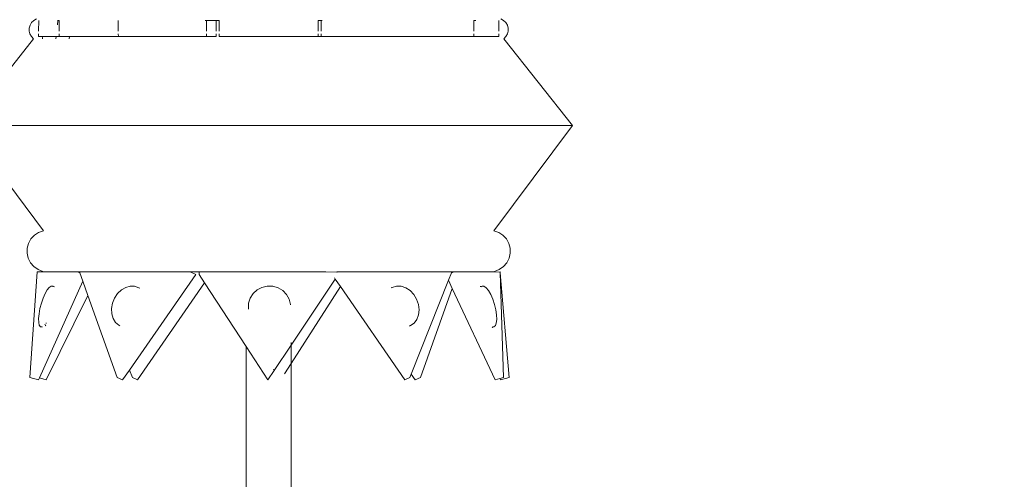
# Model space of a CAD drawing. Units: millimetres. Extents: x 7894 to 8038, y 6851 to 6951.
# Tile 39 of 49: x 7969.515 to 7972.111, y 6925.542 to 6926.755. Entities that reach past the tile are written whole.
import ezdxf

# ---------------------------------------------------------------- set-up
doc = ezdxf.new("R2010")
doc.units = ezdxf.units.MM
doc.layers.add('A-ANNO-DIMS', color=2, linetype='Continuous', lineweight=18)
doc.layers.add('A-FURN-ACCS', color=8, linetype='Continuous', lineweight=13)
doc.styles.get("Standard").update_dxf_attribs({"font": 'arial.ttf'})
doc.dimstyles.new('ISO-25', dxfattribs={"dimtxt": 1, "dimasz": 1, "dimexe": 1.25, "dimexo": 0.625, "dimtad": 1, "dimdec": 0, "dimlunit": 4, "dimtxsty": 'Standard', "dimcen": 2.5, "dimclrt": 1, "dimadec": 0, "dimazin": 0, "dimtfac": 1, "dimtdec": 0, "dimtmove": 0, "dimatfit": 3, "dimfxl": 1, "dimarcsym": 0})

# ---------------------------------------------------------------- blocks, each defined once
blk = doc.blocks.new('DISPLAY-LEAF-FINIAL-Z2_152')
for p, q in [((0.1759, 1.892, 2.1518), (0.1817, 1.8976, 2.1518)), ((0.1817, 1.8976, 2.1518), (0.1886, 1.9015, 2.1518)), ((0.1946, 1.8976, 2.1518), (0.1945, 1.8695, 2.1518)), ((0.2453, 1.8976, 2.1518), (0.2439, 1.8856, 2.1518)), ((0.2485, 1.8971, 2.1518), (0.2439, 1.8971, 2.1518)), ((0.2485, 1.8976, 2.1518), (0.2485, 1.8971, 2.1518)), ((0.2485, 1.8971, 2.1518), (0.2485, 1.8695, 2.1518)), ((0.4044, 1.8976, 2.1518), (0.4044, 1.8695, 2.1518)), ((0.6371, 1.8971, 2.1518), (0.6338, 1.8971, 2.1518)), ((0.6371, 1.8976, 2.1518), (0.6371, 1.8971, 2.1518)), ((0.6371, 1.8971, 2.1518), (0.6373, 1.8695, 2.1518)), ((0.6628, 1.8971, 2.1518), (0.6371, 1.8971, 2.1518)), ((0.6628, 1.8976, 2.1518), (0.6628, 1.8971, 2.1518)), ((0.6628, 1.8971, 2.1518), (0.6628, 1.8695, 2.1518)), ((0.6705, 1.8971, 2.1518), (0.6628, 1.8971, 2.1518)), ((0.6705, 1.8976, 2.1518), (0.6705, 1.8971, 2.1518)), ((0.6705, 1.8971, 2.1518), (0.6705, 1.8695, 2.1518)), ((0.9313, 1.8976, 2.1518), (0.9313, 1.8971, 2.1518)), ((0.9313, 1.8971, 2.1518), (0.9315, 1.8695, 2.1518)), ((0.9393, 1.8971, 2.1518), (0.9313, 1.8971, 2.1518)), ((0.9393, 1.8976, 2.1518), (0.9393, 1.8971, 2.1518)), ((0.9424, 1.8971, 2.1518), (0.9393, 1.8971, 2.1518)), ((0.9393, 1.8971, 2.1518), (0.9393, 1.8695, 2.1518)), ((1.342, 1.8976, 2.1518), (1.342, 1.8971, 2.1518)), ((1.3471, 1.8971, 2.1518), (1.342, 1.8971, 2.1518)), ((1.342, 1.8971, 2.1518), (1.3421, 1.8695, 2.1518)), ((1.4075, 1.8976, 2.1518), (1.4075, 1.8695, 2.1518)), ((1.4135, 1.9015, 2.1518), (1.4205, 1.8976, 2.1518)), ((1.4205, 1.8976, 2.1518), (1.4262, 1.892, 2.1518)), ((0.1696, 1.8695, 2.1518), (0.1697, 1.8775, 2.1518)), ((0.1715, 1.8618, 2.1518), (0.1696, 1.8695, 2.1518)), ((0.1697, 1.8775, 2.1518), (0.1719, 1.8852, 2.1518)), ((0.1719, 1.8852, 2.1518), (0.1759, 1.892, 2.1518)), ((1.4262, 1.892, 2.1518), (1.4303, 1.8852, 2.1518)), ((1.4303, 1.8852, 2.1518), (1.4325, 1.8775, 2.1518)), ((1.4326, 1.8695, 2.1518), (1.4306, 1.8618, 2.1518)), ((1.4325, 1.8775, 2.1518), (1.4326, 1.8695, 2.1518)), ((0, 1.6201, 2.1518), (0.181, 1.8491, 2.1518)), ((0.1754, 1.8548, 2.1518), (0.1715, 1.8618, 2.1518)), ((0.181, 1.8491, 2.1518), (0.1754, 1.8548, 2.1518)), ((0.1945, 1.8618, 2.1518), (0.1945, 1.8548, 2.1518)), ((0.1952, 1.8548, 2.1518), (0.1945, 1.8548, 2.1518)), ((0.2052, 1.8548, 2.1518), (0.1945, 1.8548, 2.1518)), ((0.2048, 1.8513, 2.1518), (0.2047, 1.8491, 2.1518)), ((0.2052, 1.8548, 2.1518), (0.2048, 1.8513, 2.1518)), ((0.2485, 1.8548, 2.1518), (0.2052, 1.8548, 2.1518)), ((0.2404, 1.8548, 2.1518), (0.2398, 1.8491, 2.1518)), ((0.2485, 1.8618, 2.1518), (0.2485, 1.8548, 2.1518)), ((0.2485, 1.8548, 2.1518), (0.2756, 1.8548, 2.1518)), ((0.2749, 1.8491, 2.1518), (0.2756, 1.8548, 2.1518)), ((0.2756, 1.8548, 2.1518), (0.4049, 1.8548, 2.1518)), ((0.4044, 1.8618, 2.1518), (0.4049, 1.8548, 2.1518)), ((0.4049, 1.8548, 2.1518), (0.6375, 1.8548, 2.1518)), ((0.6374, 1.8618, 2.1518), (0.6375, 1.8548, 2.1518)), ((0.6628, 1.8548, 2.1518), (0.6375, 1.8548, 2.1518)), ((0.6628, 1.8618, 2.1518), (0.6628, 1.8548, 2.1518)), ((0.6705, 1.8618, 2.1518), (0.6705, 1.8548, 2.1518)), ((0.6705, 1.8548, 2.1518), (0.9316, 1.8548, 2.1518)), ((0.9316, 1.8618, 2.1518), (0.9316, 1.8548, 2.1518)), ((0.9393, 1.8548, 2.1518), (0.9316, 1.8548, 2.1518)), ((0.9393, 1.8618, 2.1518), (0.9393, 1.8548, 2.1518)), ((1.3422, 1.8548, 2.1518), (0.9393, 1.8548, 2.1518)), ((1.3422, 1.8618, 2.1518), (1.3422, 1.8548, 2.1518)), ((1.4075, 1.8548, 2.1518), (1.3422, 1.8548, 2.1518)), ((1.4075, 1.8618, 2.1518), (1.4075, 1.8548, 2.1518)), ((1.4267, 1.8548, 2.1518), (1.4212, 1.8491, 2.1518)), ((1.4212, 1.8491, 2.1518), (1.6021, 1.6201, 2.1518)), ((1.4306, 1.8618, 2.1518), (1.4267, 1.8548, 2.1518)), ((0.2072, 1.3429, 2.1518), (0, 1.6201, 2.1518)), ((1.6021, 1.6201, 2.1518), (0, 1.6201, 2.1518)), ((1.6021, 1.6201, 2.1518), (1.395, 1.3429, 2.1518)), ((0.1742, 1.3213, 2.1518), (0.1833, 1.3311, 2.1518)), ((0.1833, 1.3311, 2.1518), (0.1945, 1.3385, 2.1518)), ((0.1945, 1.3385, 2.1518), (0.2072, 1.3429, 2.1518)), ((1.395, 1.3429, 2.1518), (1.4076, 1.3385, 2.1518)), ((1.4076, 1.3385, 2.1518), (1.4188, 1.3311, 2.1518)), ((1.4188, 1.3311, 2.1518), (1.4279, 1.3213, 2.1518)), ((0.1643, 1.2966, 2.1518), (0.1678, 1.3095, 2.1518)), ((0.1678, 1.3095, 2.1518), (0.1742, 1.3213, 2.1518)), ((1.4279, 1.3213, 2.1518), (1.4344, 1.3095, 2.1518)), ((1.4344, 1.3095, 2.1518), (1.4378, 1.2966, 2.1518)), ((0.1641, 1.2832, 2.1518), (0.1643, 1.2966, 2.1518)), ((0.1672, 1.2701, 2.1518), (0.1641, 1.2832, 2.1518)), ((1.438, 1.2832, 2.1518), (1.435, 1.2701, 2.1518)), ((1.4378, 1.2966, 2.1518), (1.438, 1.2832, 2.1518)), ((0.1733, 1.2582, 2.1518), (0.1672, 1.2701, 2.1518)), ((0.1821, 1.2481, 2.1518), (0.1733, 1.2582, 2.1518)), ((0.1931, 1.2404, 2.1518), (0.1821, 1.2481, 2.1518)), ((1.42, 1.2481, 2.1518), (1.409, 1.2404, 2.1518)), ((1.4288, 1.2582, 2.1518), (1.42, 1.2481, 2.1518)), ((1.435, 1.2701, 2.1518), (1.4288, 1.2582, 2.1518)), ((0.1714, 0.9553, 2.1518), (0.1907, 1.234, 2.1518)), ((0.2189, 1.234, 2.1518), (0.1907, 1.234, 2.1518)), ((0.2056, 1.2356, 2.1518), (0.1931, 1.2404, 2.1518)), ((0.2189, 1.234, 2.1518), (0.2056, 1.2356, 2.1518)), ((0.2189, 1.234, 2.1518), (0.2969, 1.234, 2.1518)), ((0.2969, 1.234, 2.1518), (0.3022, 1.234, 2.1518)), ((0.3029, 1.2321, 2.1518), (0.2969, 1.234, 2.1518)), ((0.3029, 1.2321, 2.1518), (0.3022, 1.234, 2.1518)), ((0.3022, 1.234, 2.1518), (0.5943, 1.234, 2.1518)), ((0.3109, 1.2098, 2.1518), (0.3029, 1.2321, 2.1518)), ((0.4339, 0.9752, 2.1518), (0.6087, 1.2276, 2.1518)), ((0.5943, 1.234, 2.1518), (0.6175, 1.234, 2.1518)), ((0.6087, 1.2276, 2.1518), (0.5943, 1.234, 2.1518)), ((0.6175, 1.2276, 2.1518), (0.6175, 1.234, 2.1518)), ((0.9517, 1.234, 2.1518), (0.6175, 1.234, 2.1518)), ((0.6322, 1.205, 2.1518), (0.6175, 1.2276, 2.1518)), ((0.9809, 1.2337, 2.1518), (0.9517, 1.234, 2.1518)), ((0.9809, 1.2337, 2.1518), (0.9815, 1.234, 2.1518)), ((0.9815, 1.234, 2.1518), (0.9829, 1.234, 2.1518)), ((1.2836, 1.234, 2.1518), (0.9829, 1.234, 2.1518)), ((1.2748, 1.2121, 2.1518), (1.2826, 1.2319, 2.1518)), ((1.2826, 1.2319, 2.1518), (1.2898, 1.234, 2.1518)), ((1.2826, 1.2319, 2.1518), (1.2836, 1.234, 2.1518)), ((1.2836, 1.234, 2.1518), (1.2898, 1.234, 2.1518)), ((1.2898, 1.234, 2.1518), (1.3832, 1.234, 2.1518)), ((1.3965, 1.2356, 2.1518), (1.3832, 1.234, 2.1518)), ((1.41, 1.2337, 2.1518), (1.3832, 1.234, 2.1518)), ((1.409, 1.2404, 2.1518), (1.3965, 1.2356, 2.1518)), ((1.4111, 1.234, 2.1518), (1.41, 1.2337, 2.1518)), ((1.4113, 1.2316, 2.1518), (1.4111, 1.234, 2.1518)), ((1.4348, 0.9553, 2.1518), (1.4113, 1.2316, 2.1518)), ((1.4203, 0.9553, 2.1518), (1.4113, 1.2316, 2.1518)), ((0.1964, 0.9543, 2.1518), (0.3109, 1.2098, 2.1518)), ((0.2227, 1.1934, 2.1518), (0.2276, 1.1967, 2.1518)), ((0.2276, 1.1967, 2.1518), (0.2317, 1.1963, 2.1518)), ((0.2325, 1.1953, 2.1518), (0.2317, 1.1963, 2.1518)), ((0.2325, 1.1953, 2.1518), (0.2366, 1.1949, 2.1518)), ((0.3244, 1.1717, 2.1518), (0.3109, 1.2098, 2.1518)), ((0.4241, 1.1934, 2.1518), (0.436, 1.1967, 2.1518)), ((0.436, 1.1967, 2.1518), (0.4475, 1.1963, 2.1518)), ((0.4475, 1.1963, 2.1518), (0.4584, 1.192, 2.1518)), ((0.455, 0.949, 2.1518), (0.6322, 1.205, 2.1518)), ((0.7416, 1.0372, 2.1518), (0.6322, 1.205, 2.1518)), ((0.7831, 1.1934, 2.1518), (0.7973, 1.1967, 2.1518)), ((0.7973, 1.1967, 2.1518), (0.8119, 1.1963, 2.1518)), ((0.8119, 1.1963, 2.1518), (0.8259, 1.1923, 2.1518)), ((0.8605, 1.0411, 2.1518), (0.9765, 1.2154, 2.1518)), ((0.8605, 0.9923, 2.1518), (0.9902, 1.1955, 2.1518)), ((0.9765, 1.2154, 2.1518), (0.9744, 1.2185, 2.1518)), ((0.9902, 1.1955, 2.1518), (0.9765, 1.2154, 2.1518)), ((1.1599, 0.949, 2.1518), (0.9902, 1.1955, 2.1518)), ((1.127, 1.1934, 2.1518), (1.1382, 1.1967, 2.1518)), ((1.1382, 1.1967, 2.1518), (1.1502, 1.1963, 2.1518)), ((1.1502, 1.1963, 2.1518), (1.1623, 1.1923, 2.1518)), ((1.1768, 0.964, 2.1518), (1.2748, 1.2121, 2.1518)), ((1.285, 1.1903, 2.1518), (1.2748, 1.2121, 2.1518)), ((1.359, 1.1953, 2.1518), (1.3638, 1.1967, 2.1518)), ((1.359, 1.1953, 2.1518), (1.3619, 1.1951, 2.1518)), ((1.3638, 1.1967, 2.1518), (1.3687, 1.1963, 2.1518)), ((1.3687, 1.1963, 2.1518), (1.3744, 1.1923, 2.1518)), ((0.2065, 1.165, 2.1518), (0.2118, 1.177, 2.1518)), ((0.2118, 1.177, 2.1518), (0.2173, 1.1867, 2.1518)), ((0.2147, 0.949, 2.1518), (0.3244, 1.1717, 2.1518)), ((0.2173, 1.1867, 2.1518), (0.2227, 1.1934, 2.1518)), ((0.4015, 0.9553, 2.1518), (0.3244, 1.1717, 2.1518)), ((0.3948, 1.165, 2.1518), (0.4028, 1.177, 2.1518)), ((0.4028, 1.177, 2.1518), (0.4128, 1.1867, 2.1518)), ((0.4128, 1.1867, 2.1518), (0.4241, 1.1934, 2.1518)), ((0.4584, 1.192, 2.1518), (0.4611, 1.1909, 2.1518)), ((0.752, 1.165, 2.1518), (0.7597, 1.177, 2.1518)), ((0.7597, 1.177, 2.1518), (0.7703, 1.1867, 2.1518)), ((0.7703, 1.1867, 2.1518), (0.7831, 1.1934, 2.1518)), ((0.8259, 1.1923, 2.1518), (0.8383, 1.1849, 2.1518)), ((0.8383, 1.1849, 2.1518), (0.8484, 1.1746, 2.1518)), ((0.8484, 1.1746, 2.1518), (0.8553, 1.1622, 2.1518)), ((1.1241, 1.1921, 2.1518), (1.1257, 1.1926, 2.1518)), ((1.1257, 1.1926, 2.1518), (1.127, 1.1934, 2.1518)), ((1.1623, 1.1923, 2.1518), (1.1737, 1.1849, 2.1518)), ((1.1737, 1.1849, 2.1518), (1.1835, 1.1746, 2.1518)), ((1.1835, 1.1746, 2.1518), (1.1911, 1.1622, 2.1518)), ((1.2015, 0.9553, 2.1518), (1.285, 1.1903, 2.1518)), ((1.398, 0.949, 2.1518), (1.285, 1.1903, 2.1518)), ((1.3744, 1.1923, 2.1518), (1.3804, 1.1849, 2.1518)), ((1.3804, 1.1849, 2.1518), (1.3863, 1.1746, 2.1518)), ((1.3863, 1.1746, 2.1518), (1.3917, 1.1622, 2.1518)), ((0.1981, 1.1374, 2.1518), (0.2018, 1.1515, 2.1518)), ((0.2018, 1.1515, 2.1518), (0.2065, 1.165, 2.1518)), ((0.3867, 1.1374, 2.1518), (0.3893, 1.1515, 2.1518)), ((0.3893, 1.1515, 2.1518), (0.3948, 1.165, 2.1518)), ((0.7475, 1.1373, 2.1518), (0.7478, 1.1515, 2.1518)), ((0.7478, 1.1515, 2.1518), (0.752, 1.165, 2.1518)), ((0.8553, 1.1622, 2.1518), (0.8587, 1.1485, 2.1518)), ((0.8587, 1.1471, 2.1518), (0.8587, 1.1485, 2.1518)), ((1.1911, 1.1622, 2.1518), (1.196, 1.1485, 2.1518)), ((1.196, 1.1485, 2.1518), (1.1978, 1.1344, 2.1518)), ((1.3917, 1.1622, 2.1518), (1.3963, 1.1485, 2.1518)), ((1.3963, 1.1485, 2.1518), (1.3997, 1.1344, 2.1518)), ((0.1943, 1.1113, 2.1518), (0.1955, 1.1237, 2.1518)), ((0.1955, 1.1237, 2.1518), (0.1981, 1.1374, 2.1518)), ((0.3871, 1.1237, 2.1518), (0.3867, 1.1374, 2.1518)), ((0.3906, 1.1113, 2.1518), (0.3871, 1.1237, 2.1518)), ((0.7474, 1.1361, 2.1518), (0.7475, 1.1373, 2.1518)), ((1.1964, 1.1209, 2.1518), (1.192, 1.1089, 2.1518)), ((1.1978, 1.1344, 2.1518), (1.1964, 1.1209, 2.1518)), ((1.3997, 1.1344, 2.1518), (1.4018, 1.1209, 2.1518)), ((1.4018, 1.1209, 2.1518), (1.4023, 1.1089, 2.1518)), ((0.1946, 1.101, 2.1518), (0.1943, 1.1113, 2.1518)), ((0.1963, 1.0936, 2.1518), (0.1946, 1.101, 2.1518)), ((0.1992, 1.0896, 2.1518), (0.1963, 1.0936, 2.1518)), ((0.2112, 1.0961, 2.1518), (0.2129, 1.0925, 2.1518)), ((0.2129, 1.0925, 2.1518), (0.2137, 1.0919, 2.1518)), ((0.2141, 1.1, 2.1518), (0.2145, 1.0978, 2.1518)), ((0.3969, 1.101, 2.1518), (0.3906, 1.1113, 2.1518)), ((0.4056, 1.0936, 2.1518), (0.3969, 1.101, 2.1518)), ((0.4087, 1.0923, 2.1518), (0.4056, 1.0936, 2.1518)), ((1.1736, 1.092, 2.1518), (1.1723, 1.0911, 2.1518)), ((1.1736, 1.092, 2.1518), (1.1752, 1.0925, 2.1518)), ((1.1847, 1.0992, 2.1518), (1.1752, 1.0925, 2.1518)), ((1.192, 1.1089, 2.1518), (1.1847, 1.0992, 2.1518)), ((1.3987, 1.0925, 2.1518), (1.3948, 1.0892, 2.1518)), ((1.4012, 1.0992, 2.1518), (1.3987, 1.0925, 2.1518)), ((1.4023, 1.1089, 2.1518), (1.4012, 1.0992, 2.1518)), ((0.2034, 1.0892, 2.1518), (0.1992, 1.0896, 2.1518)), ((0.2041, 1.0883, 2.1518), (0.2034, 1.0892, 2.1518)), ((1.3919, 1.0895, 2.1518), (1.39, 1.0879, 2.1518)), ((1.39, 1.0879, 2.1518), (1.3948, 1.0892, 2.1518)), ((0.8158, 0.974, 2.1518), (0.8605, 1.0411, 2.1518)), ((0.8605, 1.0411, 2.1518), (0.8605, 1.0475, 2.1518)), ((0.8605, 0.9923, 2.1518), (0.8605, 1.0411, 2.1518)), ((0.7416, 0, 2.1518), (0.7416, 1.0372, 2.1518)), ((0.7992, 0.949, 2.1518), (0.7416, 1.0372, 2.1518)), ((0.8431, 0.9651, 2.1518), (0.8605, 0.9923, 2.1518)), ((0.8605, 0, 2.1518), (0.8605, 0.9923, 2.1518)), ((0.4158, 0.949, 2.1518), (0.4339, 0.9752, 2.1518)), ((0.4421, 0.9553, 2.1518), (0.4339, 0.9752, 2.1518)), ((0.7992, 0.949, 2.1518), (0.8158, 0.974, 2.1518)), ((0.8158, 0.974, 2.1518), (0.8137, 0.9772, 2.1518)), ((0.8164, 0.9731, 2.1518), (0.8158, 0.974, 2.1518)), ((1.1734, 0.9553, 2.1518), (1.1768, 0.964, 2.1518)), ((1.1872, 0.949, 2.1518), (1.1768, 0.964, 2.1518)), ((0.194, 0.949, 2.1518), (0.1714, 0.9553, 2.1518)), ((0.194, 0.949, 2.1518), (0.1964, 0.9543, 2.1518)), ((0.2147, 0.949, 2.1518), (0.1964, 0.9543, 2.1518)), ((0.4158, 0.949, 2.1518), (0.4015, 0.9553, 2.1518)), ((0.455, 0.949, 2.1518), (0.4421, 0.9553, 2.1518)), ((1.1599, 0.949, 2.1518), (1.1734, 0.9553, 2.1518)), ((1.1872, 0.949, 2.1518), (1.2015, 0.9553, 2.1518)), ((1.398, 0.949, 2.1518), (1.4105, 0.9525, 2.1518)), ((1.4105, 0.9525, 2.1518), (1.4203, 0.9553, 2.1518)), ((1.412, 0.949, 2.1518), (1.4105, 0.9525, 2.1518)), ((1.412, 0.949, 2.1518), (1.4348, 0.9553, 2.1518))]:
    blk.add_line(p, q)
blk = doc.blocks.new('*D23')
at = {"layer": 'A-ANNO-DIMS', "color": 0, "lineweight": -2, "transparency": 16777216}
for p, q in [((7940.0888, 6907.098), (7940.0888, 6947.7928)), ((7971.9356, 6928.989), (7971.9356, 6947.7928)), ((7941.0888, 6946.5428), (7970.9356, 6946.5428))]:
    blk.add_line(p, q, dxfattribs=at)
at = {"layer": 'A-ANNO-DIMS', "color": 0, "transparency": 16777216}
for points in [[(7941.0888, 6946.7095), (7941.0888, 6946.3762), (7940.0888, 6946.5428)], [(7970.9356, 6946.7095), (7970.9356, 6946.3762), (7971.9356, 6946.5428)]]:
    blk.add_solid(points, dxfattribs=at)
at = {"layer": 'Defpoints', "color": 0, "transparency": 16777216}
for p in [(7971.9356, 6946.5428), (7971.9356, 6928.364), (7940.0888, 6906.473)]:
    blk.add_point(p, dxfattribs=at)
at = {"layer": 'A-ANNO-DIMS', "color": 1, "transparency": 16777216, "insert": (7956.0122, 6947.6784), "char_height": 1, "attachment_point": 5}
blk.add_mtext('2\'-8"', dxfattribs=at)
blk = doc.blocks.new('*D28')
at = {"layer": 'A-ANNO-DIMS', "color": 0, "lineweight": -2, "transparency": 16777216}
for p, q in [((7960.8854, 6936.8804), (7975.2272, 6936.8804)), ((7973.9772, 6935.8804), (7973.9772, 6923.6283)), ((7971.8421, 6922.6283), (7975.2272, 6922.6283))]:
    blk.add_line(p, q, dxfattribs=at)
at = {"layer": 'A-ANNO-DIMS', "color": 0, "transparency": 16777216}
for points in [[(7973.8105, 6935.8804), (7974.1439, 6935.8804), (7973.9772, 6936.8804)], [(7973.8105, 6923.6283), (7974.1439, 6923.6283), (7973.9772, 6922.6283)]]:
    blk.add_solid(points, dxfattribs=at)
at = {"layer": 'Defpoints', "color": 0, "transparency": 16777216}
for p in [(7960.2604, 6936.8804), (7971.2171, 6922.6283), (7973.9772, 6922.6283)]:
    blk.add_point(p, dxfattribs=at)
at = {"layer": 'A-ANNO-DIMS', "color": 1, "transparency": 16777216, "insert": (7972.8351, 6929.7543), "char_height": 1, "attachment_point": 5, "rotation": 90}
blk.add_mtext('1\'-2 1/2"', dxfattribs=at)
blk = doc.blocks.new('*D31')
at = {"layer": 'A-ANNO-DIMS', "color": 0, "lineweight": -2, "transparency": 16777216}
for p, q in [((7973.9772, 6921.7198), (7973.9772, 6926.628)), ((7949.8107, 6920.7198), (7975.2272, 6920.7198)), ((7973.9772, 6918.7198), (7973.9772, 6920.7198)), ((7950.9654, 6918.7198), (7975.2272, 6918.7198)), ((7973.9772, 6917.7198), (7973.9772, 6916.7198))]:
    blk.add_line(p, q, dxfattribs=at)
at = {"layer": 'A-ANNO-DIMS', "color": 0, "transparency": 16777216}
for points in [[(7973.8105, 6921.7198), (7974.1439, 6921.7198), (7973.9772, 6920.7198)], [(7973.8105, 6917.7198), (7974.1439, 6917.7198), (7973.9772, 6918.7198)]]:
    blk.add_solid(points, dxfattribs=at)
at = {"layer": 'Defpoints', "color": 0, "transparency": 16777216}
for p in [(7949.1857, 6920.7198), (7973.9772, 6920.7198), (7950.3404, 6918.7198)]:
    blk.add_point(p, dxfattribs=at)
at = {"layer": 'A-ANNO-DIMS', "color": 1, "transparency": 16777216, "insert": (7972.8416, 6924.6739), "char_height": 1, "attachment_point": 5, "rotation": 90}
blk.add_mtext('0\'-2"', dxfattribs=at)

msp = doc.modelspace()

# ---------------------------------------------------------------- block references
at = {"layer": 'A-FURN-ACCS'}
msp.add_blockref('DISPLAY-LEAF-FINIAL-Z2_152', (7969.3706, 6924.8555), dxfattribs=at)

# ---------------------------------------------------------------- dimensions: what is measured, and where the dimension line sits
at = {"layer": 'A-ANNO-DIMS'}
dim = msp.add_linear_dim(base=(7971.9356, 6946.5428), p1=(7940.0888, 6906.473), p2=(7971.9356, 6928.364), dimstyle='ISO-25', override={"dimdec": 1, "dimlfac": 1, "dimrnd": 0, "dimzin": 1, "dimdsep": 46, "dimlunit": 4, "dimfrac": 2}, dxfattribs=at)
dim.commit()
dim.dimension.update_dxf_attribs({"geometry": '*D23', "text_midpoint": (7956.0122, 6947.6784)})
for base, p1, p2, picture, middle in [((7973.9772, 6922.6283), (7960.2604, 6936.8804), (7971.2171, 6922.6283), '*D28', (7972.8351, 6929.7543)), ((7973.9772, 6920.7198), (7950.3404, 6918.7198), (7949.1857, 6920.7198), '*D31', (7972.8416, 6924.6739))]:
    dim = msp.add_linear_dim(base=base, p1=p1, p2=p2, angle=90, dimstyle='ISO-25', override={"dimdec": 1, "dimlfac": 1, "dimrnd": 0, "dimzin": 1, "dimdsep": 46, "dimlunit": 4, "dimfrac": 2}, dxfattribs=at)
    dim.commit()
    dim.dimension.update_dxf_attribs({"geometry": picture, "text_midpoint": middle})

doc.saveas('drawing.dxf')
